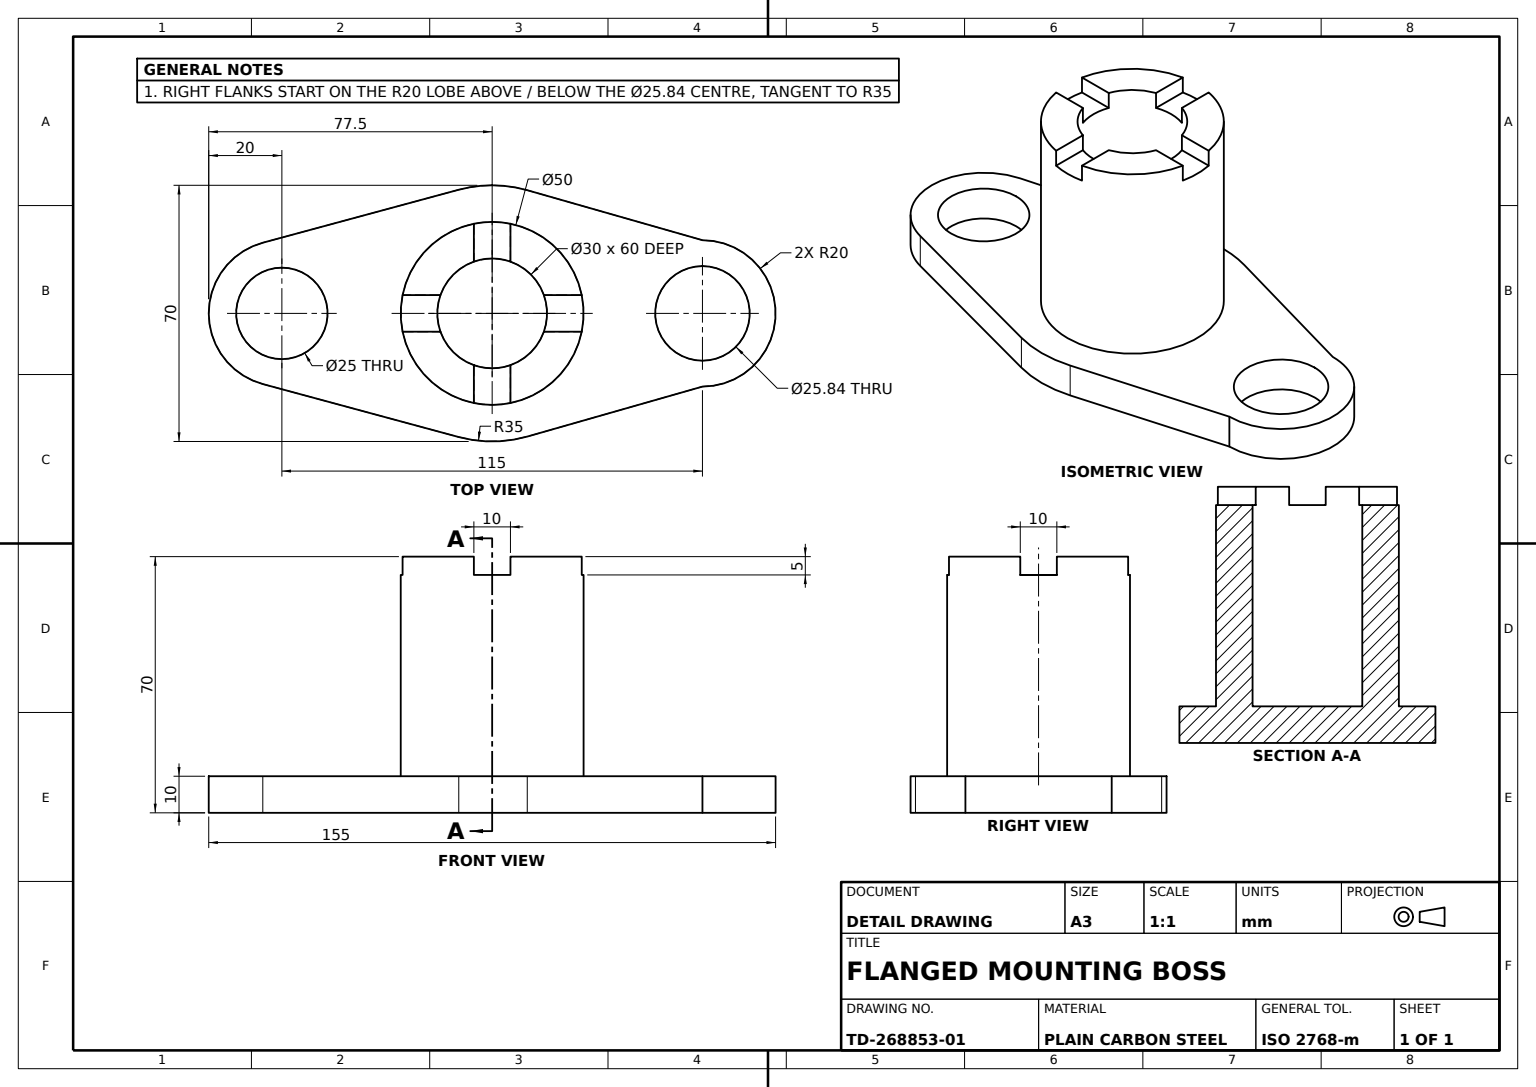
SolidWorks part; units mm, degrees
material "Plain Carbon Steel"
ref_plane "Front Plane" through (0, 0, 0) normal (0, 0, 1) x (1, 0, 0)
ref_plane "Top Plane" through (0, 0, 0) normal (0, 1, 0) x (1, 0, 0)
ref_plane "Right Plane" through (0, 0, 0) normal (1, 0, 0) x (0, 0, -1)
sketch "Flange Profile" plane through (0, 0, 0) normal (0, 1, 0) x (1, 0, 0)
  line L0 (-57.5, 0) -> (57.5, 0) construction
  line L1 (-62.7174, 19.3075) -> (-9.1304, 33.7881)
  line L2 (9.597, 33.6585) -> (57.5, 20)
  line L3 (-62.7174, -19.3075) -> (-9.1304, -33.7881)
  line L4 (9.597, -33.6585) -> (57.5, -20)
  arc A0 (-9.1304, -33.7881) -> (9.597, -33.6585) centre (0, 0) ccw
  arc A1 (-62.7174, 19.3075) -> (-62.7174, -19.3075) centre (-57.5, 0) ccw
  arc A2 (57.5, -20) -> (57.5, 20) centre (57.5, 0) ccw
  arc A3 (9.597, 33.6585) -> (-9.1304, 33.7881) centre (0, 0) ccw
  circle A4 centre (-57.5, 0) radius 12.5
  circle A5 centre (57.5, 0) radius 12.9208
  dimension "D3" = 40
  dimension "D4" = 40
  dimension "D5" = 70
  dimension "D6" = 25
  dimension "D7" = 25.8417
  dimension "D1" = 115
  dimension "D2" = 57.5
extrude "Flange Plate" add sketch "Flange Profile" along normal mid plane 10
sketch "Hub Profile" plane through (0, 5, 0) normal (0, 1, 0) x (1, 0, 0)
  line L0 (-91.3765, 0) -> (97.9943, 0) construction
  circle A0 centre (0, 0) radius 25
  circle A1 centre (0, 0) radius 15
  dimension "D1" = 50
  dimension "D2" = 30
extrude "Hub Ø50 Bore Ø30" add sketch "Hub Profile" along normal blind 60 contours A1 | A0
sketch "Cross Slot Profile" plane through (0, 65, 0) normal (0, 1, 0) x (1, 0, 0)
  line L0 (0, 49.888) -> (0, -52.9424) construction
  line L1 (-35.1252, 0) -> (39.1977, 0) construction
  line L2 (0, 35.1252) -> (0, -39.1977) construction
  line L3 (-5, 25.0621) -> (5, 25.0621)
  line L4 (-5, 25.0621) -> (-5, 14.1421)
  line L5 (-5, 14.1421) -> (5, 14.1421)
  line L6 (5, 25.0621) -> (5, 14.1421)
  line L7 (-5, 25.0621) -> (5, 14.1421) construction
  line L8 (-5, 14.1421) -> (5, 25.0621) construction
  line L9 (25.0621, 5) -> (14.1421, 5)
  line L10 (25.0621, 5) -> (25.0621, -5)
  line L11 (25.0621, -5) -> (14.1421, -5)
  line L12 (14.1421, 5) -> (14.1421, -5)
  line L13 (35.1252, 0) -> (-39.1977, 0) construction
  line L14 (5, -25.0621) -> (5, -14.1421)
  line L15 (5, -25.0621) -> (-5, -25.0621)
  line L16 (-5, -25.0621) -> (-5, -14.1421)
  line L17 (5, -14.1421) -> (-5, -14.1421)
  line L18 (0, -35.1252) -> (0, 39.1977) construction
  line L19 (-25.0621, -5) -> (-14.1421, -5)
  line L20 (-25.0621, -5) -> (-25.0621, 5)
  line L21 (-25.0621, 5) -> (-14.1421, 5)
  line L22 (-14.1421, -5) -> (-14.1421, 5)
  circle A1 centre (0, 0) radius 15 construction
  point P5 (0, 19.6021)
  point P33 (0, 0)
  dimension "D5" = 4
  dimension "D1" = 10.92
  dimension "D2" = 10
  dimension "D3" = 5
  dimension "D4" = 5
extrude "Cross Slots 4x10" cut sketch "Cross Slot Profile" against normal blind 5
